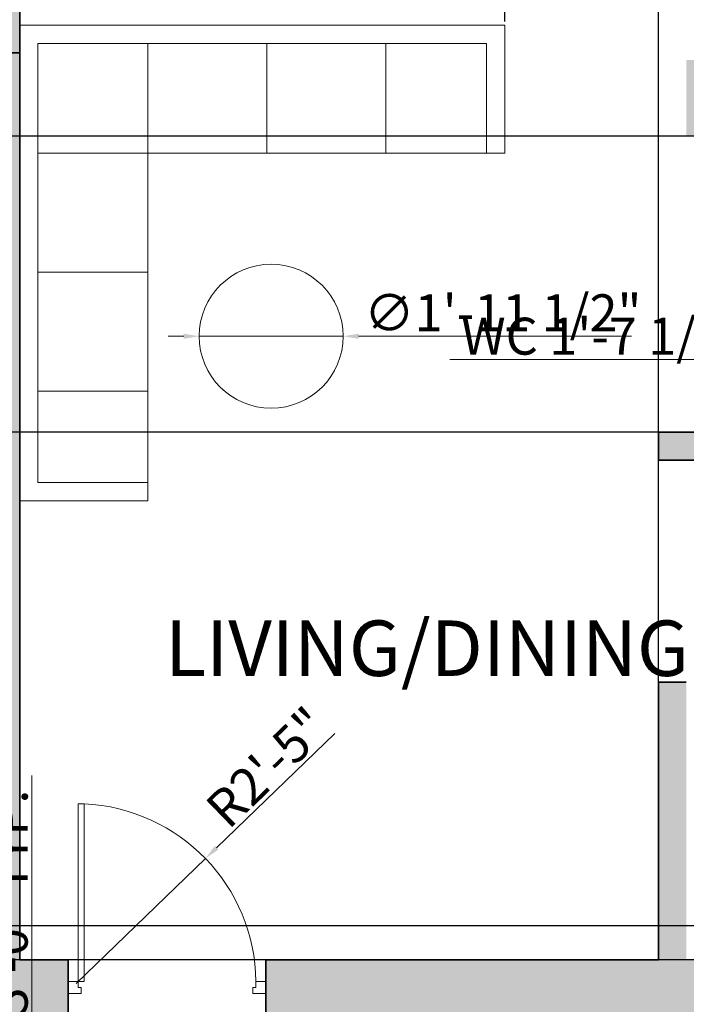
# Model space of a CAD drawing. Units: inches. Extents: x 2696 to 3240, y 1564 to 2310.
# Tile 64 of 76: x 2966 to 3074, y 1982 to 2142. Entities that reach past the tile are written whole.
import ezdxf

# ---------------------------------------------------------------- set-up
doc = ezdxf.new("R2010")
doc.units = ezdxf.units.IN
doc.linetypes.add('ACAD_ISO02W100', pattern=[15, 12, -3])
for name, color, linetype, lineweight in [('A-ANNO-DIMS', 3, 'Continuous', 18), ('A-AREA-IDEN', 7, 'Continuous', 18), ('A-DOOR', 4, 'Continuous', 18), ('A-FURN', 251, 'Continuous', 13), ('A-WALL', 7, 'Continuous', 35), ('A-WALL-OVHD', 7, 'ACAD_ISO02W100', 18), ('A-WALL-PATT', 9, 'Continuous', 13)]:
    doc.layers.add(name, color=color, linetype=linetype, lineweight=lineweight)
doc.styles.add('TIMES NEW', font='times.ttf')
doc.styles.add('YQ_DIM', font='SUPEROS.SHX', dxfattribs={"width": 0.8, "bigfont": 'HZDX.SHX'})
doc.dimstyles.new('Siddhuu', dxfattribs={"dimtxt": 6, "dimasz": 2.5, "dimexe": 1.25, "dimexo": 0.625, "dimtad": 1, "dimdec": 1, "dimlunit": 4, "dimtxsty": 'TIMES NEW', "dimcen": 2.5, "dimclrd": 256, "dimclre": 1, "dimclrt": 7, "dimadec": 0, "dimazin": 0, "dimtfac": 1, "dimtdec": 1, "dimtmove": 0, "dimatfit": 3, "dimfxl": 1, "dimtolj": 1, "dimlwd": -1, "dimarcsym": 0})

# ---------------------------------------------------------------- blocks, each defined once
blk = doc.blocks.new('DR_D01')
for p, q in [((-0.45, 0.93), (-0.42, 0.93)), ((-0.45, 0.03), (-0.45, 0.93)), ((-0.42, 0.03), (-0.42, 0.93)), ((-0.5, 0.03), (-0.42, 0.03)), ((-0.5, 0.03), (-0.5, -0.03)), ((-0.45, 0.03), (-0.45, 0)), ((-0.45, 0), (-0.435, 0)), ((-0.435, 0), (-0.435, -0.03)), ((0.435, 0), (0.435, -0.03)), ((0.45, 0), (0.435, 0)), ((0.45, 0.03), (0.45, 0)), ((0.5, 0.03), (0.45, 0.03)), ((0.5, -0.03), (0.5, 0.03)), ((-0.435, -0.03), (-0.5, -0.03)), ((0.435, -0.03), (0.5, -0.03))]:
    blk.add_line(p, q)
blk.add_arc((-0.4602, 0.0206), 0.9103, 0.5915, 87.4664)
blk = doc.blocks.new('*D30')
at = {"layer": 'A-ANNO-DIMS', "transparency": 16777216}
for p, q in [((2967.69, 1950.58), (2967.69, 2019.05)), ((2967.69, 1917.08), (2967.69, 1948.08))]:
    blk.add_line(p, q, dxfattribs=at)
at = {"layer": 'A-ANNO-DIMS', "color": 1, "lineweight": -2, "transparency": 16777216}
for p, q in [((2962.91, 1950.58), (2968.94, 1950.58)), ((2962.91, 1914.58), (2968.94, 1914.58))]:
    blk.add_line(p, q, dxfattribs=at)
at = {"layer": 'A-ANNO-DIMS', "transparency": 16777216}
for points in [[(2967.27, 1948.08), (2968.11, 1948.08), (2967.69, 1950.58)], [(2967.27, 1917.08), (2968.11, 1917.08), (2967.69, 1914.58)]]:
    blk.add_solid(points, dxfattribs=at)
at = {"layer": 'Defpoints', "color": 0, "transparency": 16777216}
for p in [(2962.29, 1950.58), (2967.69, 1950.58), (2962.29, 1914.58)]:
    blk.add_point(p, dxfattribs=at)
at = {"layer": 'A-ANNO-DIMS', "color": 7, "transparency": 16777216, "insert": (2964, 1986.06), "char_height": 6, "attachment_point": 5, "rotation": 90, "style": 'TIMES NEW'}
blk.add_mtext('\\A1;DOOR 3\'-0" TYP.', dxfattribs=at)
blk = doc.blocks.new('*D38')
at = {"layer": 'A-ANNO-DIMS', "color": 1, "lineweight": -2, "transparency": 16777216}
for p, q in [((3106.61, 2088.82), (3106.61, 2085.27)), ((3126.07, 2088.82), (3126.07, 2085.27))]:
    blk.add_line(p, q, dxfattribs=at)
at = {"layer": 'A-ANNO-DIMS', "transparency": 16777216}
for p, q in [((3106.61, 2086.52), (3035.39, 2086.52)), ((3123.57, 2086.52), (3109.11, 2086.52))]:
    blk.add_line(p, q, dxfattribs=at)
for points in [[(3109.11, 2086.94), (3109.11, 2086.11), (3106.61, 2086.52)], [(3123.57, 2086.94), (3123.57, 2086.11), (3126.07, 2086.52)]]:
    blk.add_solid(points, dxfattribs=at)
at = {"layer": 'Defpoints', "color": 0, "transparency": 16777216}
for p in [(3106.61, 2089.44), (3126.07, 2089.44), (3106.61, 2086.52)]:
    blk.add_point(p, dxfattribs=at)
at = {"layer": 'A-ANNO-DIMS', "color": 7, "transparency": 16777216, "insert": (3069.75, 2090.29), "char_height": 6, "attachment_point": 5, "style": 'TIMES NEW'}
blk.add_mtext('\\A1;WC 1\'-7 1/2" TYP.', dxfattribs=at)
blk = doc.blocks.new('*D48')
at = {"layer": 'A-ANNO-DIMS', "transparency": 16777216}
for p, q in [((3087, 1884.2), (3087, 1994.35)), ((3087, 1827.44), (3087, 1881.7))]:
    blk.add_line(p, q, dxfattribs=at)
at = {"layer": 'A-ANNO-DIMS', "color": 1, "lineweight": -2, "transparency": 16777216}
for p, q in [((3078.74, 1884.2), (3088.25, 1884.2)), ((3078.74, 1824.94), (3088.25, 1824.94))]:
    blk.add_line(p, q, dxfattribs=at)
at = {"layer": 'A-ANNO-DIMS', "transparency": 16777216}
for points in [[(3086.58, 1881.7), (3087.42, 1881.7), (3087, 1884.2)], [(3086.58, 1827.44), (3087.42, 1827.44), (3087, 1824.94)]]:
    blk.add_solid(points, dxfattribs=at)
at = {"layer": 'Defpoints', "color": 0, "transparency": 16777216}
for p in [(3078.11, 1884.2), (3087, 1884.2), (3078.11, 1824.94)]:
    blk.add_point(p, dxfattribs=at)
at = {"layer": 'A-ANNO-DIMS', "color": 7, "transparency": 16777216, "insert": (3083.23, 1940.53), "char_height": 6, "attachment_point": 5, "rotation": 90, "style": 'TIMES NEW'}
blk.add_mtext('\\A1;SECTIONAL 4\'-11 1/2" TYP.', dxfattribs=at)
blk = doc.blocks.new('*D61')
at = {"layer": 'A-ANNO-DIMS', "color": 1, "lineweight": -2, "transparency": 16777216}
for p, q in [((2965.71, 2141.33), (2965.71, 2298.45)), ((3044.3, 2141.33), (3044.3, 2298.45))]:
    blk.add_line(p, q, dxfattribs=at)
at = {"layer": 'A-ANNO-DIMS', "transparency": 16777216}
blk.add_line((2968.21, 2297.2), (3041.8, 2297.2), dxfattribs=at)
for points in [[(2968.21, 2297.62), (2968.21, 2296.78), (2965.71, 2297.2)], [(3041.8, 2297.62), (3041.8, 2296.78), (3044.3, 2297.2)]]:
    blk.add_solid(points, dxfattribs=at)
at = {"layer": 'Defpoints', "color": 0, "transparency": 16777216}
for p in [(3044.3, 2297.2), (2965.71, 2140.7), (3044.3, 2140.7)]:
    blk.add_point(p, dxfattribs=at)
at = {"layer": 'A-ANNO-DIMS', "color": 7, "transparency": 16777216, "insert": (3005.01, 2300.96), "char_height": 6, "attachment_point": 5, "style": 'TIMES NEW'}
blk.add_mtext('\\A1;6\'-6 1/2"', dxfattribs=at)
blk = doc.blocks.new('*D63')
at = {"layer": 'A-ANNO-DIMS', "color": 1, "lineweight": -2, "transparency": 16777216}
for p, q in [((2965.71, 1989.83), (2965.71, 2298.45)), ((3069.21, 1989.83), (3069.21, 2298.45))]:
    blk.add_line(p, q, dxfattribs=at)
at = {"layer": 'A-ANNO-DIMS', "transparency": 16777216}
blk.add_line((2968.21, 2297.2), (3066.71, 2297.2), dxfattribs=at)
for points in [[(2968.21, 2297.62), (2968.21, 2296.78), (2965.71, 2297.2)], [(3066.71, 2297.62), (3066.71, 2296.78), (3069.21, 2297.2)]]:
    blk.add_solid(points, dxfattribs=at)
at = {"layer": 'Defpoints', "color": 0, "transparency": 16777216}
for p in [(3069.21, 2297.2), (2965.71, 1989.2), (3069.21, 1989.2)]:
    blk.add_point(p, dxfattribs=at)
at = {"layer": 'A-ANNO-DIMS', "color": 7, "transparency": 16777216, "insert": (3017.46, 2300.96), "char_height": 6, "attachment_point": 5, "style": 'TIMES NEW'}
blk.add_mtext('\\A1;8\'-7 1/2"', dxfattribs=at)
blk = doc.blocks.new('*D64')
at = {"layer": 'A-ANNO-DIMS', "color": 1, "lineweight": -2, "transparency": 16777216}
for p, q in [((3073.08, 2206.7), (2709.36, 2206.7)), ((3068.58, 1989.2), (2709.36, 1989.2))]:
    blk.add_line(p, q, dxfattribs=at)
at = {"layer": 'A-ANNO-DIMS', "transparency": 16777216}
blk.add_line((2710.61, 1991.7), (2710.61, 2204.2), dxfattribs=at)
for points in [[(2710.19, 2204.2), (2711.03, 2204.2), (2710.61, 2206.7)], [(2710.19, 1991.7), (2711.03, 1991.7), (2710.61, 1989.2)]]:
    blk.add_solid(points, dxfattribs=at)
at = {"layer": 'Defpoints', "color": 0, "transparency": 16777216}
for p in [(2710.61, 2206.7), (3073.71, 2206.7), (3069.21, 1989.2)]:
    blk.add_point(p, dxfattribs=at)
at = {"layer": 'A-ANNO-DIMS', "color": 7, "transparency": 16777216, "insert": (2706.85, 2097.95), "char_height": 6, "attachment_point": 5, "rotation": 90, "style": 'TIMES NEW'}
blk.add_mtext('\\A1;18\'-1 1/2"', dxfattribs=at)
blk = doc.blocks.new('*D66')
at = {"layer": 'A-ANNO-DIMS', "color": 1, "lineweight": -2, "transparency": 16777216}
for p, q in [((3077.58, 2122.7), (2709.36, 2122.7)), ((3077.58, 2074.7), (2709.36, 2074.7))]:
    blk.add_line(p, q, dxfattribs=at)
at = {"layer": 'A-ANNO-DIMS', "transparency": 16777216}
blk.add_line((2710.61, 2077.2), (2710.61, 2120.2), dxfattribs=at)
for points in [[(2710.19, 2120.2), (2711.03, 2120.2), (2710.61, 2122.7)], [(2710.19, 2077.2), (2711.03, 2077.2), (2710.61, 2074.7)]]:
    blk.add_solid(points, dxfattribs=at)
at = {"layer": 'Defpoints', "color": 0, "transparency": 16777216}
for p in [(2710.61, 2122.7), (3078.21, 2122.7), (3078.21, 2074.7)]:
    blk.add_point(p, dxfattribs=at)
at = {"layer": 'A-ANNO-DIMS', "color": 7, "transparency": 16777216, "insert": (2706.93, 2098.7), "char_height": 6, "attachment_point": 5, "rotation": 90, "style": 'TIMES NEW'}
blk.add_mtext('\\A1;4\'-0"', dxfattribs=at)
blk = doc.blocks.new('*D77')
at = {"layer": 'A-ANNO-DIMS', "transparency": 16777216}
for p, q in [((2710.61, 1997.2), (2710.61, 2030.6)), ((2710.61, 1989.2), (2710.61, 1994.7)), ((2710.61, 1986.7), (2710.61, 1984.2))]:
    blk.add_line(p, q, dxfattribs=at)
at = {"layer": 'A-ANNO-DIMS', "color": 1, "lineweight": -2, "transparency": 16777216}
for p, q in [((3189.99, 1994.7), (2709.36, 1994.7)), ((3189.99, 1989.2), (2709.36, 1989.2))]:
    blk.add_line(p, q, dxfattribs=at)
at = {"layer": 'A-ANNO-DIMS', "transparency": 16777216}
for points in [[(2710.19, 1997.2), (2711.03, 1997.2), (2710.61, 1994.7)], [(2710.19, 1986.7), (2711.03, 1986.7), (2710.61, 1989.2)]]:
    blk.add_solid(points, dxfattribs=at)
at = {"layer": 'Defpoints', "color": 0, "transparency": 16777216}
for p in [(2710.61, 1994.7), (3190.61, 1994.7), (3190.61, 1989.2)]:
    blk.add_point(p, dxfattribs=at)
at = {"layer": 'A-ANNO-DIMS', "color": 7, "transparency": 16777216, "insert": (2706.85, 2015.15), "char_height": 6, "attachment_point": 5, "rotation": 90, "style": 'TIMES NEW'}
blk.add_mtext('\\A1;0\'-5 1/2"', dxfattribs=at)
blk = doc.blocks.new('*D82')
at = {"layer": 'A-ANNO-DIMS', "transparency": 16777216}
for p, q in [((2992.28, 2090.28), (2989.78, 2090.28)), ((2994.78, 2090.28), (3018.12, 2090.28)), ((3064.85, 2090.27), (3020.62, 2090.28))]:
    blk.add_line(p, q, dxfattribs=at)
for points in [[(2992.28, 2090.69), (2992.28, 2089.86), (2994.78, 2090.28)], [(3020.62, 2090.69), (3020.62, 2089.86), (3018.12, 2090.28)]]:
    blk.add_solid(points, dxfattribs=at)
at = {"layer": 'Defpoints', "color": 0, "transparency": 16777216}
for p in [(2994.78, 2090.28), (3018.12, 2090.28)]:
    blk.add_point(p, dxfattribs=at)
at = {"layer": 'A-ANNO-DIMS', "color": 7, "transparency": 16777216, "insert": (3043.98, 2094.08), "char_height": 6, "attachment_point": 5, "rotation": 359.9981, "style": 'TIMES NEW'}
blk.add_mtext('\\A1;∅1\'-11 1/2"', dxfattribs=at)
blk = doc.blocks.new('*D85')
at = {"layer": 'A-ANNO-DIMS', "transparency": 16777216}
for p, q in [((3016.79, 2025.9), (2997.6, 2007.34)), ((2974.86, 1985.36), (2995.8, 2005.61))]:
    blk.add_line(p, q, dxfattribs=at)
blk.add_solid([(2997.31, 2007.64), (2997.89, 2007.04), (2995.8, 2005.61)], dxfattribs=at)
at = {"layer": 'Defpoints', "color": 0, "transparency": 16777216}
for p in [(2995.8, 2005.61), (2974.86, 1985.36)]:
    blk.add_point(p, dxfattribs=at)
at = {"layer": 'A-ANNO-DIMS', "color": 7, "transparency": 16777216, "insert": (3005.81, 2020.4), "char_height": 6, "attachment_point": 5, "rotation": 44.0288, "style": 'TIMES NEW'}
blk.add_mtext('\\A1;R2\'-5"', dxfattribs=at)

msp = doc.modelspace()

# ---------------------------------------------------------------- hatches: boundary and pattern name
at = {"layer": 'A-WALL-PATT', "transparency": 33554556}
h = msp.add_hatch(color=256, dxfattribs=at)
h.dxf.hatch_style = 1
h.paths.add_polyline_path([(2879.11, 2253.2), (2905.91, 2253.2), (2905.91, 2262.2), (2841.89, 2262.2), (2841.89, 2253.2), (2870.11, 2253.2), (2870.11, 2176.6), (2965.71, 2176.6), (2965.71, 2206.7), (2973.58, 2206.7), (2973.58, 2215.7), (2965.71, 2215.7), (2965.71, 2262.2), (2929.91, 2262.2), (2929.91, 2253.2), (2956.71, 2253.2), (2956.71, 2185.6), (2879.11, 2185.6)])
h.paths.add_polyline_path([(2782.83, 2262.2), (2745.61, 2262.2), (2745.61, 2228.73), (2754.61, 2228.73), (2754.61, 2253.2), (2782.83, 2253.2)])
h.paths.add_polyline_path([(2754.61, 2136.2), (2965.71, 2136.2), (2965.71, 2145.2), (2879.11, 2145.2), (2879.11, 2147.07), (2877.34, 2147.07), (2870.11, 2147.07), (2870.11, 2145.2), (2754.61, 2145.2), (2754.61, 2169.67), (2745.61, 2169.67), (2745.61, 2000.2), (2754.61, 2000.2), (2754.61, 2019.2), (2849.08, 2019.2), (2849.08, 2023.7), (2841.21, 2023.7), (2841.21, 2051.83), (2836.71, 2051.83), (2836.71, 2023.7), (2754.61, 2023.7), (2754.61, 2091.2), (2836.71, 2091.2), (2836.71, 2087.83), (2841.21, 2087.83), (2841.21, 2095.7), (2754.61, 2095.7)])
h.paths.add_polyline_path([(2965.71, 2136.2), (2956.71, 2136.2), (2956.71, 2023.7), (2885.08, 2023.7), (2885.08, 2019.2), (2956.71, 2019.2), (2956.71, 1950.58), (2965.71, 1950.58), (2965.71, 1980.2), (2973.58, 1980.2), (2973.58, 1989.2), (2965.71, 1989.2)])
h.paths.add_polyline_path([(2754.61, 1906.7), (2880.21, 1906.7), (2884.71, 1906.7), (2956.71, 1906.7), (2956.71, 1792.7), (2944.71, 1792.7), (2944.71, 1783.7), (2956.71, 1783.7), (2956.71, 1740.2), (2884.71, 1740.2), (2884.71, 1783.7), (2896.71, 1783.7), (2896.71, 1792.7), (2884.71, 1792.7), (2884.71, 1846.7), (2880.21, 1846.7), (2880.21, 1740.2), (2754.61, 1740.2), (2754.61, 1777.2), (2745.61, 1777.2), (2745.61, 1692.7), (2754.61, 1692.7), (2754.61, 1731.2), (2956.71, 1731.2), (2956.71, 1723.33), (2965.71, 1723.33), (2965.71, 1884.2), (2973.58, 1884.2), (2973.58, 1893.2), (2965.71, 1893.2), (2965.71, 1914.58), (2956.71, 1914.58), (2956.71, 1911.2), (2754.61, 1911.2), (2754.61, 1930.2), (2745.61, 1930.2), (2745.61, 1817.2), (2754.61, 1817.2), (2754.61, 1854.2), (2826.61, 1854.2), (2826.61, 1868.83), (2822.11, 1868.83), (2822.11, 1858.7), (2754.61, 1858.7)])
h.paths.add_polyline_path([(2965.71, 1656.2), (3008.24, 1656.2), (3008.24, 1665.2), (2965.71, 1665.2), (2965.71, 1693.33), (2956.71, 1693.33), (2956.71, 1686.2), (2934.58, 1686.2), (2934.58, 1681.7), (2956.71, 1681.7), (2956.71, 1614.2), (2896.71, 1614.2), (2896.71, 1681.7), (2904.58, 1681.7), (2904.58, 1686.2), (2892.21, 1686.2), (2892.21, 1614.2), (2858.41, 1614.2), (2858.41, 1605.2), (2965.71, 1605.2)])
h.paths.add_polyline_path([(2788.41, 1614.2), (2754.61, 1614.2), (2754.61, 1652.7), (2745.61, 1652.7), (2745.61, 1605.2), (2788.41, 1605.2)])
h.paths.add_polyline_path([(3199.61, 1633.05), (3190.61, 1633.05), (3190.61, 1614.2), (3082.61, 1614.2), (3082.61, 1665.2), (3070.24, 1665.2), (3070.24, 1656.2), (3078.11, 1656.2), (3078.11, 1605.2), (3199.61, 1605.2)])
h.paths.add_polyline_path([(3199.61, 1702.05), (3190.61, 1702.05), (3190.61, 1699.7), (3106.61, 1699.7), (3106.61, 1747.7), (3190.61, 1747.7), (3190.61, 1752.2), (3082.61, 1752.2), (3082.61, 1760.08), (3078.11, 1760.08), (3078.11, 1747.7), (3102.11, 1747.7), (3102.11, 1699.7), (3078.11, 1699.7), (3078.11, 1695.2), (3190.61, 1695.2), (3190.61, 1676.35), (3199.61, 1676.35)])
h.paths.add_polyline_path([(3199.61, 1783.2), (3190.61, 1783.2), (3190.61, 1745.35), (3199.61, 1745.35)])
h.paths.add_polyline_path([(3082.61, 1884.2), (3190.61, 1884.2), (3190.61, 1853.2), (3199.61, 1853.2), (3199.61, 1901.7), (3190.61, 1901.7), (3190.61, 1893.2), (3005.58, 1893.2), (3005.58, 1891.28), (3005.58, 1884.2), (3078.11, 1884.2), (3078.11, 1792.08), (3082.61, 1792.08)])
h.paths.add_polyline_path([(3199.61, 1994.7), (3190.61, 1994.7), (3190.61, 1989.2), (3073.71, 1989.2), (3073.71, 2034.2), (3069.21, 2034.2), (3069.21, 1989.2), (3005.58, 1989.2), (3005.58, 1980.2), (3190.61, 1980.2), (3190.61, 1971.7), (3199.61, 1971.7)])
h.paths.add_polyline_path([(3199.61, 2155.2), (3190.61, 2155.2), (3190.61, 2064.7), (3199.61, 2064.7)])
h.paths.add_polyline_path([(3190.61, 2074.7), (3106.61, 2074.7), (3106.61, 2122.7), (3190.61, 2122.7), (3190.61, 2127.2), (3082.71, 2127.2), (3082.71, 2135.08), (3073.71, 2135.08), (3073.71, 2122.7), (3102.11, 2122.7), (3102.11, 2074.7), (3069.21, 2074.7), (3069.21, 2070.2), (3190.61, 2070.2)])
h.paths.add_polyline_path([(3082.71, 2253.2), (3190.61, 2253.2), (3190.61, 2225.2), (3199.61, 2225.2), (3199.61, 2262.2), (3073.71, 2262.2), (3073.71, 2215.7), (3035.58, 2215.7), (3035.58, 2206.7), (3073.71, 2206.7), (3073.71, 2171.08), (3082.71, 2171.08)])

# ---------------------------------------------------------------- linework, layer by layer
at = {"layer": 'A-FURN'}
for p, q in [((2965.71, 2140.7), (3044.3, 2140.7)), ((2965.71, 2063.59), (2965.71, 2140.7)), ((3044.3, 2140.7), (3044.3, 2119.94)), ((2968.67, 2066.56), (2968.67, 2137.74)), ((2968.67, 2137.74), (3041.34, 2137.74)), ((2986.47, 2063.59), (2986.47, 2137.74)), ((3005.75, 2119.94), (3005.75, 2137.74)), ((3025.02, 2119.94), (3025.02, 2137.74)), ((3041.34, 2137.74), (3041.34, 2119.94)), ((2968.67, 2119.94), (3044.3, 2119.94)), ((2968.67, 2100.66), (2986.47, 2100.66)), ((2968.67, 2081.39), (2986.47, 2081.39)), ((2986.47, 2066.56), (2968.67, 2066.56)), ((2986.47, 2063.59), (2965.71, 2063.59))]:
    msp.add_line(p, q, dxfattribs=at)
msp.add_circle((3006.45, 2090.28), 11.67, dxfattribs=at)
at = {"layer": 'A-WALL'}
for p, q in [((2965.71, 2145.2), (2965.71, 2136.2)), ((2754.61, 2136.2), (2965.71, 2136.2)), ((2965.71, 2136.2), (2965.71, 1989.2)), ((3069.21, 2074.7), (3102.11, 2074.7)), ((3069.21, 2074.7), (3069.21, 2070.2)), ((3069.21, 2070.2), (3190.61, 2070.2)), ((3069.21, 2034.2), (3069.21, 1989.2)), ((3069.21, 2034.2), (3073.71, 2034.2)), ((2965.71, 1989.2), (2973.58, 1989.2)), ((2973.58, 1980.2), (2973.58, 1989.2)), ((3005.58, 1989.2), (3069.21, 1989.2)), ((3005.58, 1980.2), (3005.58, 1989.2))]:
    msp.add_line(p, q, dxfattribs=at)
at = {"layer": 'A-WALL-OVHD'}
msp.add_line((3069.21, 2034.2), (3069.21, 2070.2), dxfattribs=at)

# ---------------------------------------------------------------- block references
at = {"layer": 'A-DOOR', "xscale": 32, "yscale": 32, "zscale": 32}
msp.add_blockref('DR_D01', (2989.58, 1984.7), dxfattribs=at)

# ---------------------------------------------------------------- texts
at = {"layer": 'A-AREA-IDEN', "insert": (2989.23, 2044.2), "char_height": 9, "attachment_point": 1, "style": 'YQ_DIM'}
msp.add_mtext_dynamic_manual_height_columns('LIVING/DINING', width=92.6128, gutter_width=12.5, heights=[0], dxfattribs=at)

# ---------------------------------------------------------------- dimensions: what is measured, and where the dimension line sits
at = {"layer": 'A-ANNO-DIMS'}
for base, p1, p2, picture, middle in [((3044.3, 2297.2), (2965.71, 2140.7), (3044.3, 2140.7), '*D61', (3005.01, 2300.96)), ((3069.21, 2297.2), (2965.71, 1989.2), (3069.21, 1989.2), '*D63', (3017.46, 2300.96))]:
    dim = msp.add_linear_dim(base=base, p1=p1, p2=p2, dimstyle='Siddhuu', override={"dimdec": 1, "dimlfac": 1, "dimrnd": 0, "dimzin": 1, "dimdsep": 46, "dimlunit": 4, "dimfrac": 2}, dxfattribs=at)
    dim.commit()
    dim.dimension.update_dxf_attribs({"geometry": picture, "text_midpoint": middle})
for base, p1, p2, picture, middle in [((2710.61, 2206.7), (3069.21, 1989.2), (3073.71, 2206.7), '*D64', (2706.85, 2097.95)), ((2710.61, 2122.7), (3078.21, 2074.7), (3078.21, 2122.7), '*D66', (2706.93, 2098.7)), ((2710.61, 1994.7), (3190.61, 1989.2), (3190.61, 1994.7), '*D77', (2706.85, 2015.15))]:
    dim = msp.add_linear_dim(base=base, p1=p1, p2=p2, angle=90, dimstyle='Siddhuu', override={"dimdec": 1, "dimlfac": 1, "dimrnd": 0, "dimzin": 1, "dimdsep": 46, "dimlunit": 4, "dimfrac": 2}, dxfattribs=at)
    dim.commit()
    dim.dimension.update_dxf_attribs({"geometry": picture, "text_midpoint": middle})
for base, p1, p2, angle, text, picture, middle in [((3106.61, 2086.52), (3126.07, 2089.44), (3106.61, 2089.44), 180, 'WC <> TYP.', '*D38', (3069.75, 2090.29)), ((2967.69, 1950.58), (2962.29, 1914.58), (2962.29, 1950.58), 90, 'DOOR <> TYP.', '*D30', (2964, 1986.06)), ((3087, 1884.2), (3078.11, 1824.94), (3078.11, 1884.2), 90, 'SECTIONAL <> TYP.', '*D48', (3083.23, 1940.53))]:
    dim = msp.add_linear_dim(base=base, p1=p1, p2=p2, angle=angle, text=text, dimstyle='Siddhuu', override={"dimdec": 1, "dimlfac": 1, "dimrnd": 0, "dimzin": 1, "dimdsep": 46, "dimlunit": 4, "dimfrac": 2}, dxfattribs=at)
    dim.commit()
    dim.dimension.update_dxf_attribs({"geometry": picture, "text_midpoint": middle})
dim = msp.add_diameter_dim_2p(p1=(2994.78, 2090.28), p2=(3018.12, 2090.28), dimstyle='Siddhuu', override={"dimdec": 1, "dimlfac": 1, "dimrnd": 0, "dimzin": 1, "dimdsep": 46, "dimlunit": 4, "dimfrac": 2}, dxfattribs=at)
dim.commit()
dim.dimension.update_dxf_attribs({"geometry": '*D82', "text_midpoint": (3043.98, 2090.28), "dimtype": 163})
dim = msp.add_radius_dim(center=(2974.86, 1985.36), mpoint=(2995.8, 2005.61), dimstyle='Siddhuu', override={"dimdec": 1, "dimlfac": 1, "dimrnd": 0, "dimzin": 1, "dimdsep": 46, "dimlunit": 4, "dimfrac": 2}, dxfattribs=at)
dim.commit()
dim.dimension.update_dxf_attribs({"geometry": '*D85', "text_midpoint": (3008.36, 2017.75), "dimtype": 164})

doc.saveas('drawing.dxf')
